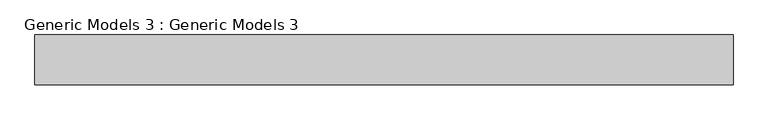
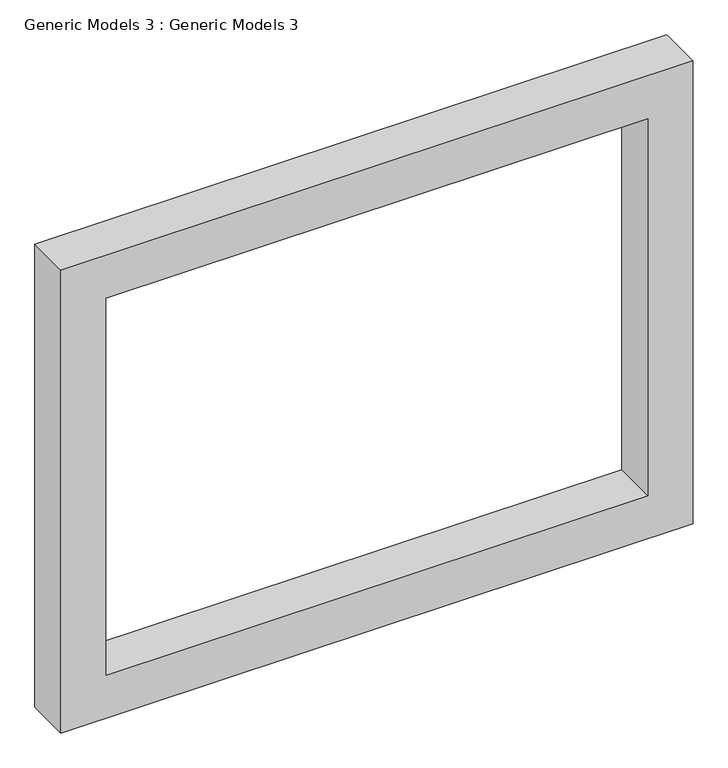
"""IFC4 building model written with IfcOpenShell, lengths in millimetres: proxy geometry, Generic Models 3 : Generic Models 3."""

from ifc_helpers import new_model, si_unit, frame, origin, place, context, project, spatial, polyline, outline, extrude, source, transform, mapped, element, save


def generic_models_3_generic_models_3_1617b94e(model_context):
    return source(origin(), model_context, "Body", "SweptSolid", [
        extrude(outline(polyline([(2717.8, -1945.1328791), (2717.8, -4078.7328791), (1066.8, -4078.7328791), (1066.8, -1945.1328791), (2717.8, -1945.1328791)]), holes=[polyline([(2565.4, -2097.5328791), (1219.2, -2097.5328791), (1219.2, -3926.3328791), (2565.4, -3926.3328791), (2565.4, -2097.5328791)])]), frame((0.0, -2602.2776789, 0.0), z_axis=(0.0, 1.0, 0.0), x_axis=(0.0, 0.0, 1.0)), (0.0, 0.0, 1.0), 152.4),
    ])


if __name__ == "__main__":
    model = new_model("IFC4")
    model_context = context("Model", 3, world=origin())
    ifc_project = project(units=[si_unit("LENGTHUNIT", "METRE", prefix="MILLI")], contexts=[model_context])
    site = spatial("IfcSite", under=ifc_project)
    building = spatial("IfcBuilding", under=site)
    placement = place(None, origin())
    generic_models_3_generic_models_3_shape = generic_models_3_generic_models_3_1617b94e(model_context)
    element("IfcBuildingElementProxy", 1, Name="Generic Models 3 : Generic Models 3", ObjectType="Generic Models 3 : Generic Models 3", at=placement, inside=building, context=model_context, shape_type="MappedRepresentation", body=[
        mapped(generic_models_3_generic_models_3_shape, transform((0.0, 0.0, 0.0), x_axis=(1.0, 0.0, 0.0), y_axis=(0.0, 1.0, 0.0), z_axis=(0.0, 0.0, 1.0))),
    ])
    save(model, "model.ifc")

# Revit data of these elements
# Element 1 (IfcBuildingElementProxy, "Generic Models 3 : Generic Models 3")
#   Materials on its faces: "WALNUT WOOD COLOUR 5\""
# Materials
#   "WALNUT WOOD COLOUR 5\"": class "Generic", colour RGB 120 120 120, transparency 0, Cost = 0
